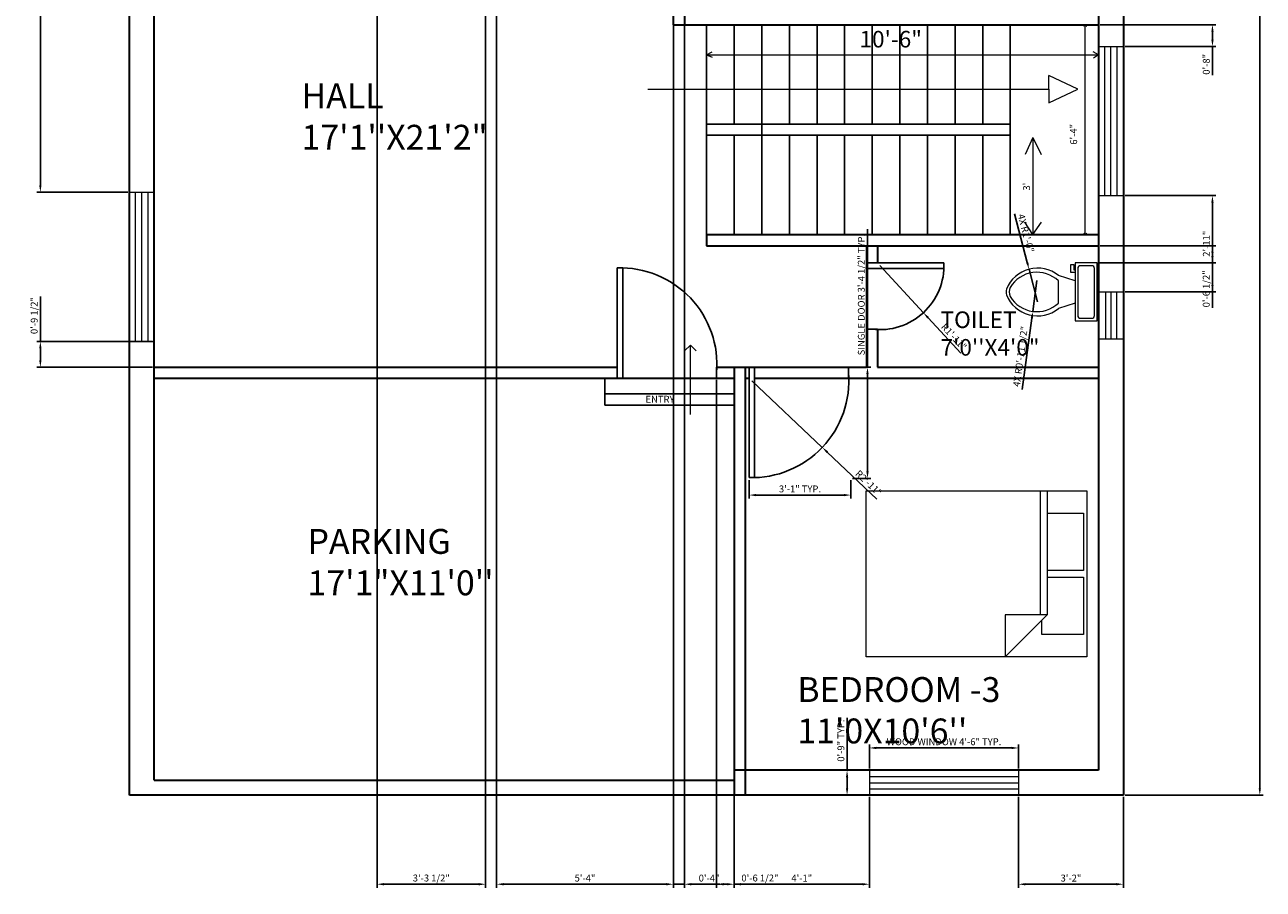
# Model space of a CAD drawing. Units: inches. Extents: x 2572 to 3021, y 1553 to 2232.
# Tile 1 of 3: x 2572 to 3021, y 1553 to 1866. Entities that reach past the tile are written whole.
import ezdxf

# ---------------------------------------------------------------- set-up
doc = ezdxf.new("R2010")
doc.units = ezdxf.units.IN
for name, color, linetype, lineweight in [('A-ANNO-DIMS', 2, 'Continuous', 18), ('A-ANNO-SYMB', 3, 'Continuous', 18), ('A-ANNO-TEXT', 7, 'Continuous', 18), ('A-AREA-IDEN', 7, 'Continuous', 25), ('A-DOOR', 3, 'Continuous', 25), ('A-FLOR-FIXT', 9, 'Continuous', 18), ('A-FLOR-STRS', 7, 'Continuous', 25), ('A-FURN', 8, 'Continuous', 18), ('A-GLAZ', 4, 'Continuous', 18), ('A-WALL', 7, 'Continuous', 35)]:
    doc.layers.add(name, color=color, linetype=linetype, lineweight=lineweight)
doc.styles.get("Standard").update_dxf_attribs({"font": 'arial.ttf'})
doc.dimstyles.new('ISO-25', dxfattribs={"dimtxt": 2.5, "dimasz": 2.5, "dimexe": 1.25, "dimexo": 0.625, "dimtad": 1, "dimdec": 1, "dimlunit": 3, "dimtxsty": 'Standard', "dimcen": 2.5, "dimadec": 0, "dimazin": 0, "dimtfac": 1, "dimtdec": 1, "dimtmove": 0, "dimatfit": 3, "dimfxl": 1, "dimarcsym": 0})

# ---------------------------------------------------------------- blocks, each defined once
blk = doc.blocks.new('Toilet - top')
for p, q in [((9.5, -6), (9.5, -2)), ((-10, -8.5), (-8, -8.5)), ((-10, -9.5), (-10, -8.5)), ((-8, -8.5), (-8, -8)), ((-7, -8), (-7, -9.5)), ((-4, -8), (-6, -14)), ((4, -8), (6, -14)), ((-7, -9.5), (-10, -9.5)), ((4, -14), (-4, -14))]:
    blk.add_line(p, q)
blk.add_lwpolyline([(10.5, -8), (10.5, 0), (-10.5, 0), (-10.5, -8)], close=True)
for points in [[(-9.5, -2), (-9.5, -6)], [(8.5, -1), (-8.5, -1)], [(-8.5, -7), (8.5, -7)]]:
    blk.add_lwpolyline(points)
for centre, radius, start, end in [((-8.62, -1.88), 0.884, 81.8699, 188.1301), ((8.62, -1.88), 0.884, 351.8699, 98.1301), ((-8.62, -6.12), 0.884, 171.8699, 278.1301), ((8.62, -6.12), 0.884, 261.8699, 8.1301), ((3.52, -21.58), 12.17, 141.4691, 247.9714), ((4.2, -21.82), 11.33, 136.3677, 238.9468), ((-3.52, -21.58), 12.17, 292.0284, 38.5307), ((-4.2, -21.82), 11.33, 301.053, 43.6321), ((0, -27.88), 4, 245.7318, 294.2682), ((0, -29), 4, 254.8605, 285.1395)]:
    blk.add_arc(centre, radius, start, end)
blk = doc.blocks.new('Bed - Queen')
for p, q in [((0, -80.00003), (0, 0)), ((0, 0), (59.99999, 0)), ((59.99999, 0), (59.99999, -80.00003)), ((7.99999, -1.2), (28.79998, -1.2)), ((7.99999, -14.4), (7.99999, -1.2)), ((28.79998, -1.2), (28.79998, -14.4)), ((31.19999, -1.2), (51.99999, -1.2)), ((31.19999, -14.4), (31.19999, -1.2)), ((51.99999, -1.2), (51.99999, -16.4)), ((0, -14.4), (44.8, -14.4)), ((44.8, -16.8), (0, -16.8)), ((59.99999, -29.6), (44.8, -14.4)), ((44.8, -14.4), (44.8, -29.6)), ((51.99999, -16.4), (46.79936, -16.4)), ((44.8, -29.6), (59.99999, -29.6)), ((59.99999, -80.00003), (0, -80.00003))]:
    blk.add_line(p, q)
blk = doc.blocks.new('Window - Wood Frame 36 in. Wide plan')
for p, q in [((0, 6), (0, 0)), ((36, 6), (36, 0)), ((0, 4.5), (36, 4.5)), ((0, 3), (36, 3)), ((0, 1.5), (36, 1.5))]:
    blk.add_line(p, q)
blk = doc.blocks.new('*D6')
at = {"layer": 'A-ANNO-DIMS', "color": 0, "lineweight": -2, "transparency": 16777216}
for p, q in [((2970.8, 2187.37), (3020.83, 2187.37)), ((3019.58, 2184.87), (3019.58, 1589.87)), ((2970.8, 1587.37), (3020.83, 1587.37))]:
    blk.add_line(p, q, dxfattribs=at)
at = {"layer": 'A-ANNO-DIMS', "color": 0, "transparency": 16777216}
for points in [[(3019.16, 2184.87), (3019.99, 2184.87), (3019.58, 2187.37)], [(3019.16, 1589.87), (3019.99, 1589.87), (3019.58, 1587.37)]]:
    blk.add_solid(points, dxfattribs=at)
at = {"layer": 'Defpoints', "color": 0, "transparency": 16777216}
for p in [(2970.18, 2187.37), (2970.18, 1587.37), (3019.58, 1587.37)]:
    blk.add_point(p, dxfattribs=at)
at = {"layer": 'A-ANNO-DIMS', "color": 0, "transparency": 16777216, "insert": (3014.36, 1887.37), "char_height": 9, "attachment_point": 5, "rotation": 90}
blk.add_mtext("50'", dxfattribs=at)
blk = doc.blocks.new('DOOR-SINGLE-36IN')
for p, q in [((0, 40.01), (0, 36.01)), ((0, 36.01), (0, 0.01)), ((2, 0.01), (2, 40.01)), ((36, 40.01), (36, 36.01)), ((0, 0.01), (2, 0.01))]:
    blk.add_line(p, q)
blk.add_arc((1, 35.12), 35.12, 268.3683, 4.728)
blk = doc.blocks.new('WIN-BATH-17IN')
for p, q in [((0, 17), (9, 17)), ((2.5, 17), (2.5, 0)), ((4.5, 17), (4.5, 0)), ((6.5, 17), (6.5, 0)), ((0, 0), (9, 0))]:
    blk.add_line(p, q)
blk = doc.blocks.new('*D10')
at = {"layer": 'A-ANNO-DIMS', "color": 0, "lineweight": -2, "transparency": 16777216}
for p, q in [((2878.2, 1597), (2878.2, 1605.72)), ((2880.7, 1604.47), (2929.7, 1604.47)), ((2932.2, 1597), (2932.2, 1605.72))]:
    blk.add_line(p, q, dxfattribs=at)
at = {"layer": 'A-ANNO-DIMS', "color": 0, "transparency": 16777216}
for points in [[(2880.7, 1604.89), (2880.7, 1604.06), (2878.2, 1604.47)], [(2929.7, 1604.89), (2929.7, 1604.06), (2932.2, 1604.47)]]:
    blk.add_solid(points, dxfattribs=at)
at = {"layer": 'Defpoints', "color": 0, "transparency": 16777216}
for p in [(2932.2, 1604.47), (2878.2, 1596.37), (2932.2, 1596.37)]:
    blk.add_point(p, dxfattribs=at)
at = {"layer": 'A-ANNO-DIMS', "color": 0, "transparency": 16777216, "insert": (2905.2, 1606.39), "char_height": 2.5, "attachment_point": 5}
blk.add_mtext('WOOD WINDOW 4\'-6" TYP.', dxfattribs=at)
blk = doc.blocks.new('*D11')
at = {"layer": 'A-ANNO-DIMS', "color": 0, "lineweight": -2, "transparency": 16777216}
for p, q in [((2870.1, 1596.37), (2870.1, 1615.36)), ((2877.58, 1596.37), (2868.85, 1596.37)), ((2870.1, 1589.87), (2870.1, 1593.87)), ((2877.58, 1587.37), (2868.85, 1587.37))]:
    blk.add_line(p, q, dxfattribs=at)
at = {"layer": 'A-ANNO-DIMS', "color": 0, "transparency": 16777216}
for points in [[(2869.69, 1593.87), (2870.52, 1593.87), (2870.1, 1596.37)], [(2869.69, 1589.87), (2870.52, 1589.87), (2870.1, 1587.37)]]:
    blk.add_solid(points, dxfattribs=at)
at = {"layer": 'Defpoints', "color": 0, "transparency": 16777216}
for p in [(2870.1, 1596.37), (2878.2, 1596.37), (2878.2, 1587.37)]:
    blk.add_point(p, dxfattribs=at)
at = {"layer": 'A-ANNO-DIMS', "color": 0, "transparency": 16777216, "insert": (2868.2, 1607.12), "char_height": 2.5, "attachment_point": 5, "rotation": 90}
blk.add_mtext('0\'-9" TYP.', dxfattribs=at)
blk = doc.blocks.new('*D16')
at = {"layer": 'A-ANNO-DIMS', "color": 0, "lineweight": -2, "transparency": 16777216}
for p, q in [((2877.5, 1742.37), (2877.5, 1792.4)), ((2872.08, 1742.37), (2878.75, 1742.37)), ((2877.5, 1704.59), (2877.5, 1739.87)), ((2872.08, 1702.09), (2878.75, 1702.09))]:
    blk.add_line(p, q, dxfattribs=at)
at = {"layer": 'A-ANNO-DIMS', "color": 0, "transparency": 16777216}
for points in [[(2877.08, 1739.87), (2877.91, 1739.87), (2877.5, 1742.37)], [(2877.08, 1704.59), (2877.91, 1704.59), (2877.5, 1702.09)]]:
    blk.add_solid(points, dxfattribs=at)
at = {"layer": 'Defpoints', "color": 0, "transparency": 16777216}
for p in [(2871.45, 1742.37), (2877.5, 1742.37), (2871.45, 1702.09)]:
    blk.add_point(p, dxfattribs=at)
at = {"layer": 'A-ANNO-DIMS', "color": 0, "transparency": 16777216, "insert": (2875.58, 1768.64), "char_height": 2.5, "attachment_point": 5, "rotation": 90}
blk.add_mtext('SINGLE DOOR 3\'-4 1/2" TYP.', dxfattribs=at)
blk = doc.blocks.new('*D17')
at = {"layer": 'A-ANNO-DIMS', "color": 0, "lineweight": -2, "transparency": 16777216}
for p, q in [((2834.63, 1701.46), (2834.63, 1694.8)), ((2871.45, 1701.46), (2871.45, 1694.8)), ((2837.13, 1696.05), (2868.95, 1696.05))]:
    blk.add_line(p, q, dxfattribs=at)
at = {"layer": 'A-ANNO-DIMS', "color": 0, "transparency": 16777216}
for points in [[(2837.13, 1696.46), (2837.13, 1695.63), (2834.63, 1696.05)], [(2868.95, 1696.46), (2868.95, 1695.63), (2871.45, 1696.05)]]:
    blk.add_solid(points, dxfattribs=at)
at = {"layer": 'Defpoints', "color": 0, "transparency": 16777216}
for p in [(2834.63, 1702.09), (2871.45, 1702.09), (2871.45, 1696.05)]:
    blk.add_point(p, dxfattribs=at)
at = {"layer": 'A-ANNO-DIMS', "color": 0, "transparency": 16777216, "insert": (2853.04, 1697.95), "char_height": 2.5, "attachment_point": 5}
blk.add_mtext('3\'-1" TYP.', dxfattribs=at)
blk = doc.blocks.new('*D22')
at = {"layer": 'A-ANNO-DIMS', "color": 0, "lineweight": -2, "transparency": 16777216}
for p, q in [((2932.2, 1586.75), (2932.2, 1553.87)), ((2970.18, 1586.75), (2970.18, 1553.87)), ((2934.7, 1555.12), (2967.68, 1555.12))]:
    blk.add_line(p, q, dxfattribs=at)
at = {"layer": 'A-ANNO-DIMS', "color": 0, "transparency": 16777216}
for points in [[(2934.7, 1555.54), (2934.7, 1554.7), (2932.2, 1555.12)], [(2967.68, 1555.54), (2967.68, 1554.7), (2970.18, 1555.12)]]:
    blk.add_solid(points, dxfattribs=at)
at = {"layer": 'Defpoints', "color": 0, "transparency": 16777216}
for p in [(2932.2, 1587.37), (2970.18, 1587.37), (2970.18, 1555.12)]:
    blk.add_point(p, dxfattribs=at)
at = {"layer": 'A-ANNO-DIMS', "color": 0, "transparency": 16777216, "insert": (2951.19, 1557.02), "char_height": 2.5, "attachment_point": 5}
blk.add_mtext('3\'-2"', dxfattribs=at)
blk = doc.blocks.new('*D24')
at = {"layer": 'A-ANNO-DIMS', "color": 0, "lineweight": -2, "transparency": 16777216}
for p, q in [((2618.55, 1986.37), (2576.67, 1986.37)), ((2577.92, 1983.87), (2577.92, 1808.21)), ((2609.55, 1805.71), (2576.67, 1805.71))]:
    blk.add_line(p, q, dxfattribs=at)
at = {"layer": 'A-ANNO-DIMS', "color": 0, "transparency": 16777216}
for points in [[(2577.51, 1983.87), (2578.34, 1983.87), (2577.92, 1986.37)], [(2577.51, 1808.21), (2578.34, 1808.21), (2577.92, 1805.71)]]:
    blk.add_solid(points, dxfattribs=at)
at = {"layer": 'Defpoints', "color": 0, "transparency": 16777216}
for p in [(2619.18, 1986.37), (2577.92, 1805.71), (2610.18, 1805.71)]:
    blk.add_point(p, dxfattribs=at)
at = {"layer": 'A-ANNO-DIMS', "color": 0, "transparency": 16777216, "insert": (2576, 1896.04), "char_height": 2.5, "attachment_point": 5, "rotation": 90}
blk.add_mtext('15\'-0 1/2"', dxfattribs=at)
blk = doc.blocks.new('*D28')
at = {"layer": 'A-ANNO-DIMS', "color": 0, "lineweight": -2, "transparency": 16777216}
for p, q in [((2961.8, 1866.37), (3003.68, 1866.37)), ((3002.43, 1863.87), (3002.43, 1861)), ((2970.8, 1858.5), (3003.68, 1858.5)), ((3002.43, 1858.5), (3002.43, 1848.1))]:
    blk.add_line(p, q, dxfattribs=at)
at = {"layer": 'A-ANNO-DIMS', "color": 0, "transparency": 16777216}
for points in [[(3002.02, 1863.87), (3002.85, 1863.87), (3002.43, 1866.37)], [(3002.02, 1861), (3002.85, 1861), (3002.43, 1858.5)]]:
    blk.add_solid(points, dxfattribs=at)
at = {"layer": 'Defpoints', "color": 0, "transparency": 16777216}
for p in [(2961.18, 1866.37), (2970.18, 1858.5), (3002.43, 1858.5)]:
    blk.add_point(p, dxfattribs=at)
at = {"layer": 'A-ANNO-DIMS', "color": 0, "transparency": 16777216, "insert": (3000.53, 1852.05), "char_height": 2.5, "attachment_point": 5, "rotation": 90}
blk.add_mtext('0\'-8"', dxfattribs=at)
blk = doc.blocks.new('*D29')
at = {"layer": 'A-ANNO-DIMS', "color": 0, "lineweight": -2, "transparency": 16777216}
for p, q in [((2970.8, 1804.5), (3003.68, 1804.5)), ((3002.43, 1802), (3002.43, 1772.16)), ((2970.8, 1769.66), (3003.68, 1769.66))]:
    blk.add_line(p, q, dxfattribs=at)
at = {"layer": 'A-ANNO-DIMS', "color": 0, "transparency": 16777216}
for points in [[(3002.02, 1802), (3002.85, 1802), (3002.43, 1804.5)], [(3002.02, 1772.16), (3002.85, 1772.16), (3002.43, 1769.66)]]:
    blk.add_solid(points, dxfattribs=at)
at = {"layer": 'Defpoints', "color": 0, "transparency": 16777216}
for p in [(2970.18, 1804.5), (2970.18, 1769.66), (3002.43, 1769.66)]:
    blk.add_point(p, dxfattribs=at)
at = {"layer": 'A-ANNO-DIMS', "color": 0, "transparency": 16777216, "insert": (3000.55, 1787.08), "char_height": 2.5, "attachment_point": 5, "rotation": 90}
blk.add_mtext('2\'-11"', dxfattribs=at)
blk = doc.blocks.new('*D35')
at = {"layer": 'A-ANNO-DIMS', "color": 0, "lineweight": -2, "transparency": 16777216}
for p, q in [((2807.18, 1995.31), (2807.18, 1553.87)), ((2743.18, 1985.75), (2743.18, 1553.87)), ((2745.68, 1555.12), (2804.68, 1555.12))]:
    blk.add_line(p, q, dxfattribs=at)
at = {"layer": 'A-ANNO-DIMS', "color": 0, "transparency": 16777216}
for points in [[(2745.68, 1555.54), (2745.68, 1554.7), (2743.18, 1555.12)], [(2804.68, 1555.54), (2804.68, 1554.7), (2807.18, 1555.12)]]:
    blk.add_solid(points, dxfattribs=at)
at = {"layer": 'Defpoints', "color": 0, "transparency": 16777216}
for p in [(2807.18, 1995.94), (2743.18, 1986.37), (2807.18, 1555.12)]:
    blk.add_point(p, dxfattribs=at)
at = {"layer": 'A-ANNO-DIMS', "color": 0, "transparency": 16777216, "insert": (2775.18, 1557.02), "char_height": 2.5, "attachment_point": 5}
blk.add_mtext('5\'-4"', dxfattribs=at)
blk = doc.blocks.new('*D36')
at = {"layer": 'A-ANNO-DIMS', "color": 0, "lineweight": -2, "transparency": 16777216}
for p, q in [((2822.85, 1737.75), (2822.85, 1553.87)), ((2829.18, 1737.75), (2829.18, 1553.87)), ((2825.35, 1555.12), (2826.68, 1555.12)), ((2829.18, 1555.12), (2845.4, 1555.12))]:
    blk.add_line(p, q, dxfattribs=at)
at = {"layer": 'A-ANNO-DIMS', "color": 0, "transparency": 16777216}
for points in [[(2825.35, 1555.54), (2825.35, 1554.7), (2822.85, 1555.12)], [(2826.68, 1555.54), (2826.68, 1554.7), (2829.18, 1555.12)]]:
    blk.add_solid(points, dxfattribs=at)
at = {"layer": 'Defpoints', "color": 0, "transparency": 16777216}
for p in [(2822.85, 1738.37), (2829.18, 1738.37), (2829.18, 1555.12)]:
    blk.add_point(p, dxfattribs=at)
at = {"layer": 'A-ANNO-DIMS', "color": 0, "transparency": 16777216, "insert": (2838.54, 1557.04), "char_height": 2.5, "attachment_point": 5}
blk.add_mtext('0\'-6 1/2"', dxfattribs=at)
blk = doc.blocks.new('*D38')
at = {"layer": 'A-ANNO-DIMS', "color": 0, "lineweight": -2, "transparency": 16777216}
for p, q in [((2699.85, 2177.75), (2699.85, 1553.87)), ((2739.18, 2177.75), (2739.18, 1553.87)), ((2736.68, 1555.12), (2702.35, 1555.12))]:
    blk.add_line(p, q, dxfattribs=at)
at = {"layer": 'A-ANNO-DIMS', "color": 0, "transparency": 16777216}
for points in [[(2702.35, 1555.54), (2702.35, 1554.7), (2699.85, 1555.12)], [(2736.68, 1555.54), (2736.68, 1554.7), (2739.18, 1555.12)]]:
    blk.add_solid(points, dxfattribs=at)
at = {"layer": 'Defpoints', "color": 0, "transparency": 16777216}
for p in [(2699.85, 2178.37), (2739.18, 2178.37), (2699.85, 1555.12)]:
    blk.add_point(p, dxfattribs=at)
at = {"layer": 'A-ANNO-DIMS', "color": 0, "transparency": 16777216, "insert": (2719.51, 1557.04), "char_height": 2.5, "attachment_point": 5}
blk.add_mtext('3\'-3 1/2"', dxfattribs=at)
blk = doc.blocks.new('*D39')
at = {"layer": 'A-ANNO-DIMS', "color": 0, "lineweight": -2, "transparency": 16777216}
for p, q in [((2807.18, 2177.75), (2807.18, 1553.87)), ((2811.18, 2177.75), (2811.18, 1553.87)), ((2804.68, 1555.12), (2802.18, 1555.12)), ((2807.18, 1555.12), (2811.18, 1555.12)), ((2813.68, 1555.12), (2824.07, 1555.12))]:
    blk.add_line(p, q, dxfattribs=at)
at = {"layer": 'A-ANNO-DIMS', "color": 0, "transparency": 16777216}
for points in [[(2804.68, 1555.54), (2804.68, 1554.7), (2807.18, 1555.12)], [(2813.68, 1555.54), (2813.68, 1554.7), (2811.18, 1555.12)]]:
    blk.add_solid(points, dxfattribs=at)
at = {"layer": 'Defpoints', "color": 0, "transparency": 16777216}
for p in [(2807.18, 2178.37), (2811.18, 2178.37), (2811.18, 1555.12)]:
    blk.add_point(p, dxfattribs=at)
at = {"layer": 'A-ANNO-DIMS', "color": 0, "transparency": 16777216, "insert": (2820.12, 1557.02), "char_height": 2.5, "attachment_point": 5}
blk.add_mtext('0\'-4"', dxfattribs=at)
blk = doc.blocks.new('*D41')
at = {"layer": 'A-ANNO-DIMS', "color": 0, "lineweight": -2, "transparency": 16777216}
for p, q in [((2829.18, 1586.75), (2829.18, 1553.87)), ((2878.2, 1586.75), (2878.2, 1553.87)), ((2831.68, 1555.12), (2875.7, 1555.12))]:
    blk.add_line(p, q, dxfattribs=at)
at = {"layer": 'A-ANNO-DIMS', "color": 0, "transparency": 16777216}
for points in [[(2831.68, 1555.54), (2831.68, 1554.7), (2829.18, 1555.12)], [(2875.7, 1555.54), (2875.7, 1554.7), (2878.2, 1555.12)]]:
    blk.add_solid(points, dxfattribs=at)
at = {"layer": 'Defpoints', "color": 0, "transparency": 16777216}
for p in [(2829.18, 1587.37), (2878.2, 1587.37), (2878.2, 1555.12)]:
    blk.add_point(p, dxfattribs=at)
at = {"layer": 'A-ANNO-DIMS', "color": 0, "transparency": 16777216, "insert": (2853.69, 1557), "char_height": 2.5, "attachment_point": 5}
blk.add_mtext('4\'-1"', dxfattribs=at)
blk = doc.blocks.new('*D42')
at = {"layer": 'A-ANNO-DIMS', "color": 0, "lineweight": -2, "transparency": 16777216}
for p, q in [((2577.92, 1751.71), (2577.92, 1767.93)), ((2618.55, 1751.71), (2576.67, 1751.71)), ((2577.92, 1744.87), (2577.92, 1749.21)), ((2618.55, 1742.37), (2576.67, 1742.37))]:
    blk.add_line(p, q, dxfattribs=at)
at = {"layer": 'A-ANNO-DIMS', "color": 0, "transparency": 16777216}
for points in [[(2577.51, 1749.21), (2578.34, 1749.21), (2577.92, 1751.71)], [(2577.51, 1744.87), (2578.34, 1744.87), (2577.92, 1742.37)]]:
    blk.add_solid(points, dxfattribs=at)
at = {"layer": 'Defpoints', "color": 0, "transparency": 16777216}
for p in [(2577.92, 1751.71), (2619.18, 1751.71), (2619.18, 1742.37)]:
    blk.add_point(p, dxfattribs=at)
at = {"layer": 'A-ANNO-DIMS', "color": 0, "transparency": 16777216, "insert": (2576, 1761.07), "char_height": 2.5, "attachment_point": 5, "rotation": 90}
blk.add_mtext('0\'-9 1/2"', dxfattribs=at)
blk = doc.blocks.new('*D46')
at = {"layer": 'A-ANNO-DIMS', "color": 0, "lineweight": -2, "transparency": 16777216}
for p, q in [((2961.8, 1786.37), (3003.68, 1786.37)), ((3002.43, 1783.87), (3002.43, 1782.61)), ((2961.3, 1780.11), (3003.68, 1780.11)), ((3002.43, 1780.11), (3002.43, 1763.89))]:
    blk.add_line(p, q, dxfattribs=at)
at = {"layer": 'A-ANNO-DIMS', "color": 0, "transparency": 16777216}
for points in [[(3002.02, 1783.87), (3002.85, 1783.87), (3002.43, 1786.37)], [(3002.02, 1782.61), (3002.85, 1782.61), (3002.43, 1780.11)]]:
    blk.add_solid(points, dxfattribs=at)
at = {"layer": 'Defpoints', "color": 0, "transparency": 16777216}
for p in [(2961.18, 1786.37), (2960.68, 1780.11), (3002.43, 1780.11)]:
    blk.add_point(p, dxfattribs=at)
at = {"layer": 'A-ANNO-DIMS', "color": 0, "transparency": 16777216, "insert": (3000.51, 1770.75), "char_height": 2.5, "attachment_point": 5, "rotation": 90}
blk.add_mtext('0\'-6 1/2"', dxfattribs=at)
blk = doc.blocks.new('*D47')
at = {"layer": 'A-ANNO-DIMS', "color": 0, "lineweight": -2, "transparency": 16777216}
for p, q in [((2835.63, 1737.48), (2861.12, 1713.33)), ((2880.86, 1694.63), (2862.94, 1711.61))]:
    blk.add_line(p, q, dxfattribs=at)
at = {"layer": 'A-ANNO-DIMS', "color": 0, "transparency": 16777216}
blk.add_solid([(2863.23, 1711.91), (2862.65, 1711.3), (2861.12, 1713.33)], dxfattribs=at)
at = {"layer": 'Defpoints', "color": 0, "transparency": 16777216}
for p in [(2835.63, 1737.48), (2861.12, 1713.33)]:
    blk.add_point(p, dxfattribs=at)
at = {"layer": 'A-ANNO-DIMS', "color": 0, "transparency": 16777216, "insert": (2877.71, 1700.2), "char_height": 2.5, "attachment_point": 5, "rotation": 316.5482}
blk.add_mtext('R2\'-11"', dxfattribs=at)
blk = doc.blocks.new('*D51')
at = {"layer": 'A-ANNO-DIMS', "color": 0, "lineweight": -2, "transparency": 16777216}
for p, q in [((2882.02, 1779.14), (2897.74, 1762.11)), ((2911.32, 1747.4), (2899.44, 1760.27))]:
    blk.add_line(p, q, dxfattribs=at)
at = {"layer": 'A-ANNO-DIMS', "color": 0, "transparency": 16777216}
blk.add_solid([(2899.74, 1760.55), (2899.13, 1759.99), (2897.74, 1762.11)], dxfattribs=at)
at = {"layer": 'Defpoints', "color": 0, "transparency": 16777216}
for p in [(2882.02, 1779.14), (2897.74, 1762.11)]:
    blk.add_point(p, dxfattribs=at)
at = {"layer": 'A-ANNO-DIMS', "color": 0, "transparency": 16777216, "insert": (2908.56, 1753.17), "char_height": 2.5, "attachment_point": 5, "rotation": 312.7085}
blk.add_mtext('R1\'-11"', dxfattribs=at)
blk = doc.blocks.new('*D52')
at = {"layer": 'A-ANNO-DIMS', "color": 0, "lineweight": -2, "transparency": 16777216}
for p, q in [((2930.73, 1797.94), (2935.37, 1780.28)), ((2939.1, 1766.09), (2936, 1777.86))]:
    blk.add_line(p, q, dxfattribs=at)
at = {"layer": 'A-ANNO-DIMS', "color": 0, "transparency": 16777216}
blk.add_solid([(2935.77, 1780.38), (2934.97, 1780.17), (2936, 1777.86)], dxfattribs=at)
at = {"layer": 'Defpoints', "color": 0, "transparency": 16777216}
for p in [(2936, 1777.86), (2939.1, 1766.09)]:
    blk.add_point(p, dxfattribs=at)
at = {"layer": 'A-ANNO-DIMS', "color": 0, "transparency": 16777216, "insert": (2934.57, 1790.8), "char_height": 2.5, "attachment_point": 5, "rotation": 284.7192}
blk.add_mtext('4X R1\'-0"', dxfattribs=at)
blk = doc.blocks.new('*D53')
at = {"layer": 'A-ANNO-DIMS', "color": 0, "lineweight": -2, "transparency": 16777216}
for p, q in [((2938.86, 1773.81), (2937.35, 1762.58)), ((2933.55, 1734.31), (2937.02, 1760.1))]:
    blk.add_line(p, q, dxfattribs=at)
at = {"layer": 'A-ANNO-DIMS', "color": 0, "transparency": 16777216}
blk.add_solid([(2936.6, 1760.16), (2937.43, 1760.05), (2937.35, 1762.58)], dxfattribs=at)
at = {"layer": 'Defpoints', "color": 0, "transparency": 16777216}
for p in [(2938.86, 1773.81), (2937.35, 1762.58)]:
    blk.add_point(p, dxfattribs=at)
at = {"layer": 'A-ANNO-DIMS', "color": 0, "transparency": 16777216, "insert": (2933.21, 1746.22), "char_height": 2.5, "attachment_point": 5, "rotation": 82.3391}
blk.add_mtext('4X R0\'-11 1/2"', dxfattribs=at)

msp = doc.modelspace()

# ---------------------------------------------------------------- linework, layer by layer
at = {"layer": 'A-ANNO-DIMS'}
for p, q in [((2956.35, 1866.37), (2955.77, 1865.82)), ((2956.35, 1790.37), (2956.35, 1866.37)), ((2956.35, 1866.37), (2956.89, 1865.81)), ((2819.22, 1855.49), (2821.3, 1856.55)), ((2819.22, 1855.49), (2961.18, 1855.49)), ((2819.22, 1855.49), (2821.3, 1854.68)), ((2961.18, 1855.49), (2959.27, 1856.56)), ((2961.18, 1855.49), (2959.34, 1854.22)), ((2937.37, 1825.52), (2934.55, 1819.41)), ((2937.37, 1825.52), (2937.37, 1790.37)), ((2937.37, 1825.52), (2940.36, 1819.41)), ((2937.37, 1790.37), (2934.5, 1794.84)), ((2937.37, 1790.37), (2940.47, 1794.84)), ((2956.35, 1790.37), (2955.89, 1790.9)), ((2956.35, 1790.37), (2956.95, 1790.9))]:
    msp.add_line(p, q, dxfattribs=at)
at = {"layer": 'A-ANNO-SYMB'}
for p, q in [((2943.2, 1843.06), (2943.2, 1848.06)), ((2953.72, 1843.02), (2943.2, 1848.06)), ((2797.99, 1843.06), (2943.2, 1843.06)), ((2943.2, 1843.06), (2943.2, 1838.06)), ((2943.2, 1838.06), (2953.72, 1843.02)), ((2813.39, 1750.39), (2811.21, 1748.24)), ((2811.21, 1748.24), (2813.39, 1750.39)), ((2813.39, 1725.25), (2813.39, 1750.39)), ((2813.39, 1750.39), (2815.49, 1748.24))]:
    msp.add_line(p, q, dxfattribs=at)
at = {"layer": 'A-DOOR'}
for p, q in [((2877.18, 1780.14), (2881.18, 1780.14)), ((2905.18, 1778.14), (2877.18, 1778.14)), ((2881.18, 1780.14), (2905.18, 1780.14)), ((2905.18, 1780.14), (2905.18, 1778.14)), ((2877.18, 1756.14), (2881.18, 1756.14))]:
    msp.add_line(p, q, dxfattribs=at)
msp.add_arc((2882.02, 1779.14), 23.18, 262.9457, 2.473, dxfattribs=at)
at = {"layer": 'A-FLOR-STRS'}
for p, q in [((2819.22, 1866.37), (2819.22, 1790.37)), ((2829.22, 1866.37), (2829.22, 1830.37)), ((2839.22, 1866.37), (2839.22, 1790.37)), ((2849.22, 1866.37), (2849.22, 1830.37)), ((2859.22, 1866.37), (2859.22, 1830.37)), ((2869.22, 1866.37), (2869.22, 1830.37)), ((2879.22, 1866.37), (2879.22, 1830.37)), ((2889.22, 1866.37), (2889.22, 1830.37)), ((2899.22, 1866.37), (2899.22, 1830.37)), ((2909.22, 1866.37), (2909.22, 1830.37)), ((2919.22, 1866.37), (2919.22, 1830.37)), ((2929.22, 1866.37), (2929.22, 1826.37)), ((2819.22, 1830.37), (2929.22, 1830.37)), ((2819.22, 1826.37), (2929.22, 1826.37)), ((2829.22, 1826.37), (2829.22, 1790.37)), ((2849.22, 1826.37), (2849.22, 1790.37)), ((2859.22, 1826.37), (2859.22, 1790.37)), ((2869.22, 1826.37), (2869.22, 1790.37)), ((2879.22, 1826.37), (2879.22, 1790.37)), ((2889.22, 1826.37), (2889.22, 1790.37)), ((2899.22, 1826.37), (2899.22, 1790.37)), ((2909.22, 1826.37), (2909.22, 1790.37)), ((2919.22, 1826.37), (2919.22, 1790.37)), ((2929.22, 1826.37), (2929.22, 1790.37)), ((2782.36, 1738.37), (2782.36, 1732.66)), ((2782.36, 1732.66), (2829.18, 1732.66)), ((2782.36, 1732.66), (2782.36, 1728.61)), ((2782.36, 1728.61), (2829.18, 1728.61))]:
    msp.add_line(p, q, dxfattribs=at)
at = {"layer": 'A-WALL'}
for p, q in [((2610.18, 1587.37), (2610.18, 2187.37)), ((2970.18, 2187.37), (2970.18, 1587.37)), ((2619.18, 1592.85), (2619.18, 2178.37)), ((2961.18, 2178.37), (2961.18, 1596.37)), ((2807.18, 1866.37), (2807.18, 2117.62)), ((2807.18, 1866.37), (2961.18, 1866.37)), ((2811.18, 1870.37), (2811.18, 1866.37)), ((2819.22, 1790.37), (2961.18, 1790.37)), ((2819.22, 1790.37), (2819.22, 1786.37)), ((2819.22, 1786.37), (2961.18, 1786.37)), ((2877.18, 1786.37), (2877.18, 1742.37)), ((2881.18, 1786.37), (2881.18, 1780.14)), ((2881.18, 1756.14), (2881.18, 1742.37)), ((2619.18, 1742.37), (2786.85, 1742.37)), ((2822.85, 1742.37), (2829.18, 1742.37)), ((2829.18, 1742.37), (2829.18, 1587.37)), ((2829.18, 1742.37), (2877.18, 1742.37)), ((2833.18, 1742.37), (2833.18, 1587.37)), ((2881.18, 1742.37), (2961.18, 1742.37)), ((2619.18, 1738.37), (2829.18, 1738.37)), ((2833.18, 1738.37), (2834.63, 1738.37)), ((2836.63, 1738.37), (2961.18, 1738.37)), ((2619.18, 1592.85), (2829.18, 1592.85)), ((2961.18, 1596.37), (2829.18, 1596.37)), ((2970.18, 1587.37), (2610.18, 1587.37))]:
    msp.add_line(p, q, dxfattribs=at)

# ---------------------------------------------------------------- block references
at = {"layer": 'A-DOOR', "extrusion": (0, 0, -1), "zscale": -1, "rotation": 180}
msp.add_blockref('DOOR-SINGLE-36IN', (-2786.85, 1778.39), dxfattribs=at)
at = {"layer": 'A-DOOR'}
msp.add_blockref('DOOR-SINGLE-36IN', (2834.63, 1702.36), dxfattribs=at)
at = {"layer": 'A-FLOR-FIXT', "rotation": 270}
msp.add_blockref('Toilet - top', (2960.68, 1769.61), dxfattribs=at)
at = {"layer": 'A-FURN', "rotation": 270}
msp.add_blockref('Bed - Queen', (2956.98, 1697.53), dxfattribs=at)
at = {"layer": 'A-GLAZ', "xscale": 1.5, "yscale": 1.5, "zscale": 1.5, "rotation": 90}
for p in [(2970.18, 1804.5), (2619.18, 1751.71)]:
    msp.add_blockref('Window - Wood Frame 36 in. Wide plan', p, dxfattribs=at)
at = {"layer": 'A-GLAZ'}
msp.add_blockref('WIN-BATH-17IN', (2961.18, 1752.66), dxfattribs=at)
at = {"layer": 'A-GLAZ', "xscale": 1.5, "yscale": 1.5, "zscale": 1.5}
msp.add_blockref('Window - Wood Frame 36 in. Wide plan', (2878.2, 1587.37), dxfattribs=at)

# ---------------------------------------------------------------- texts
at = {"layer": 'A-ANNO-DIMS', "insert": (2874.6, 1864.15), "char_height": 6, "attachment_point": 1}
msp.add_mtext_dynamic_manual_height_columns('10\'-6"', width=6, gutter_width=12.5, heights=[0], dxfattribs=at)
at = {"layer": 'A-ANNO-DIMS', "insert": (2950.94, 1822.92), "char_height": 2.5, "attachment_point": 1, "rotation": 91.1222}
msp.add_mtext('6\'-4"', dxfattribs=at)
at = {"layer": 'A-ANNO-DIMS', "insert": (2933.88, 1806.32), "char_height": 2.5, "width": 6.8156, "attachment_point": 1, "rotation": 91.1222}
msp.add_mtext("3'", dxfattribs=at)
at = {"layer": 'A-ANNO-TEXT', "insert": (2797.11, 1732.01), "char_height": 2.5, "attachment_point": 1}
msp.add_mtext_dynamic_manual_height_columns('ENTRY', width=0.9706, gutter_width=12.5, heights=[0], dxfattribs=at)
at = {"layer": 'A-AREA-IDEN', "attachment_point": 1}
for s, width, insert, char_height in [('\\pxt12;HALL                  \\P\\ptz;17\'1\'\'X21\'2"', 94.3643, (2672.51, 1845.15), 9), ('TOILET\\P7\'0\'\'X4\'0"', 2.3965, (2903.96, 1762.55), 6), ('\\pxt12;PARKING                     \\P\\ptz;17\'1"X11\'0\'\'', 94.3643, (2674.68, 1683.77), 9), ("\\pxt12;BEDROOM -3                    \\P\\ptz;11'0X10'6''", 94.3643, (2852.08, 1630.13), 9)]:
    msp.add_mtext_dynamic_manual_height_columns(s, width=width, gutter_width=12.5, heights=[0], dxfattribs=dict(at, insert=insert, char_height=char_height))

# ---------------------------------------------------------------- dimensions: what is measured, and where the dimension line sits
at = {"layer": 'A-ANNO-DIMS'}
for base, p1, p2, override, picture, middle in [((3019.58, 1587.37), (2970.18, 2187.37), (2970.18, 1587.37), {"dimtxt": 9, "dimclrd": 0, "dimclre": 0, "dimclrt": 0}, '*D6', (3014.36, 1887.37)), ((2577.92, 1805.71), (2619.18, 1986.37), (2610.18, 1805.71), {"dimdec": 1, "dimlfac": 1, "dimrnd": 0, "dimzin": 1, "dimdsep": 46, "dimlunit": 4, "dimfrac": 2}, '*D24', (2576, 1896.04)), ((3002.43, 1858.5), (2961.18, 1866.37), (2970.18, 1858.5), {"dimdec": 1, "dimlfac": 1, "dimrnd": 0, "dimzin": 1, "dimdsep": 46, "dimlunit": 4, "dimfrac": 2}, '*D28', (3000.53, 1852.05)), ((3002.43, 1769.66), (2970.18, 1804.5), (2970.18, 1769.66), {"dimdec": 1, "dimlfac": 1, "dimrnd": 0, "dimzin": 1, "dimdsep": 46, "dimlunit": 4, "dimfrac": 2}, '*D29', (3000.55, 1787.08)), ((3002.43, 1780.11), (2961.18, 1786.37), (2960.68, 1780.11), {"dimdec": 1, "dimlfac": 1, "dimrnd": 0, "dimzin": 1, "dimdsep": 46, "dimlunit": 4, "dimfrac": 2}, '*D46', (3000.51, 1770.75)), ((2577.92, 1751.71), (2619.18, 1742.37), (2619.18, 1751.71), {"dimdec": 1, "dimlfac": 1, "dimrnd": 0, "dimzin": 1, "dimdsep": 46, "dimlunit": 4, "dimfrac": 2}, '*D42', (2576, 1761.07))]:
    dim = msp.add_linear_dim(base=base, p1=p1, p2=p2, angle=90, dimstyle='ISO-25', override=override, dxfattribs=at)
    dim.commit()
    dim.dimension.update_dxf_attribs({"geometry": picture, "text_midpoint": middle})
for base, p1, p2, picture, middle in [((2699.85, 1555.12), (2739.18, 2178.37), (2699.85, 2178.37), '*D38', (2719.51, 1557.04)), ((2811.18, 1555.12), (2807.18, 2178.37), (2811.18, 2178.37), '*D39', (2820.12, 1557.02)), ((2807.18, 1555.12), (2743.18, 1986.37), (2807.18, 1995.94), '*D35', (2775.18, 1557.02)), ((2829.18, 1555.12), (2822.85, 1738.37), (2829.18, 1738.37), '*D36', (2838.54, 1557.04)), ((2878.2, 1555.12), (2829.18, 1587.37), (2878.2, 1587.37), '*D41', (2853.69, 1557)), ((2970.18, 1555.12), (2932.2, 1587.37), (2970.18, 1587.37), '*D22', (2951.19, 1557.02))]:
    dim = msp.add_linear_dim(base=base, p1=p1, p2=p2, dimstyle='ISO-25', override={"dimdec": 1, "dimlfac": 1, "dimrnd": 0, "dimzin": 1, "dimdsep": 46, "dimlunit": 4, "dimfrac": 2}, dxfattribs=at)
    dim.commit()
    dim.dimension.update_dxf_attribs({"geometry": picture, "text_midpoint": middle})
for center, mpoint, picture, middle in [((2939.1, 1766.09), (2936, 1777.86), '*D52', (2934.57, 1790.8)), ((2938.86, 1773.81), (2937.35, 1762.58), '*D53', (2933.21, 1746.22))]:
    dim = msp.add_radius_dim(center=center, mpoint=mpoint, text='4X <>', dimstyle='ISO-25', override={"dimdec": 1, "dimlfac": 1, "dimrnd": 0, "dimzin": 1, "dimdsep": 46, "dimlunit": 4, "dimfrac": 2}, dxfattribs=at)
    dim.commit()
    dim.dimension.update_dxf_attribs({"geometry": picture, "text_midpoint": middle})
for base, p1, p2, text, picture, middle in [((2877.5, 1742.37), (2871.45, 1702.09), (2871.45, 1742.37), 'SINGLE DOOR <> TYP.', '*D16', (2875.58, 1768.64)), ((2870.1, 1596.37), (2878.2, 1587.37), (2878.2, 1596.37), '<> TYP.', '*D11', (2868.2, 1607.12))]:
    dim = msp.add_linear_dim(base=base, p1=p1, p2=p2, angle=90, text=text, dimstyle='ISO-25', override={"dimdec": 1, "dimlfac": 1, "dimrnd": 0, "dimzin": 1, "dimdsep": 46, "dimlunit": 4, "dimfrac": 2}, dxfattribs=at)
    dim.commit()
    dim.dimension.update_dxf_attribs({"geometry": picture, "text_midpoint": middle})
for center, mpoint, picture, middle in [((2882.02, 1779.14), (2897.74, 1762.11), '*D51', (2907.17, 1751.89)), ((2835.63, 1737.48), (2861.12, 1713.33), '*D47', (2876.42, 1698.83))]:
    dim = msp.add_radius_dim(center=center, mpoint=mpoint, dimstyle='ISO-25', override={"dimdec": 1, "dimlfac": 1, "dimrnd": 0, "dimzin": 1, "dimdsep": 46, "dimlunit": 4, "dimfrac": 2}, dxfattribs=at)
    dim.commit()
    dim.dimension.update_dxf_attribs({"geometry": picture, "text_midpoint": middle, "dimtype": 164})
for base, p1, p2, text, picture, middle in [((2871.45, 1696.05), (2834.63, 1702.09), (2871.45, 1702.09), '<> TYP.', '*D17', (2853.04, 1697.95)), ((2932.2, 1604.47), (2878.2, 1596.37), (2932.2, 1596.37), 'WOOD WINDOW <> TYP.', '*D10', (2905.2, 1606.39))]:
    dim = msp.add_linear_dim(base=base, p1=p1, p2=p2, text=text, dimstyle='ISO-25', override={"dimdec": 1, "dimlfac": 1, "dimrnd": 0, "dimzin": 1, "dimdsep": 46, "dimlunit": 4, "dimfrac": 2}, dxfattribs=at)
    dim.commit()
    dim.dimension.update_dxf_attribs({"geometry": picture, "text_midpoint": middle})

doc.saveas('drawing.dxf')
